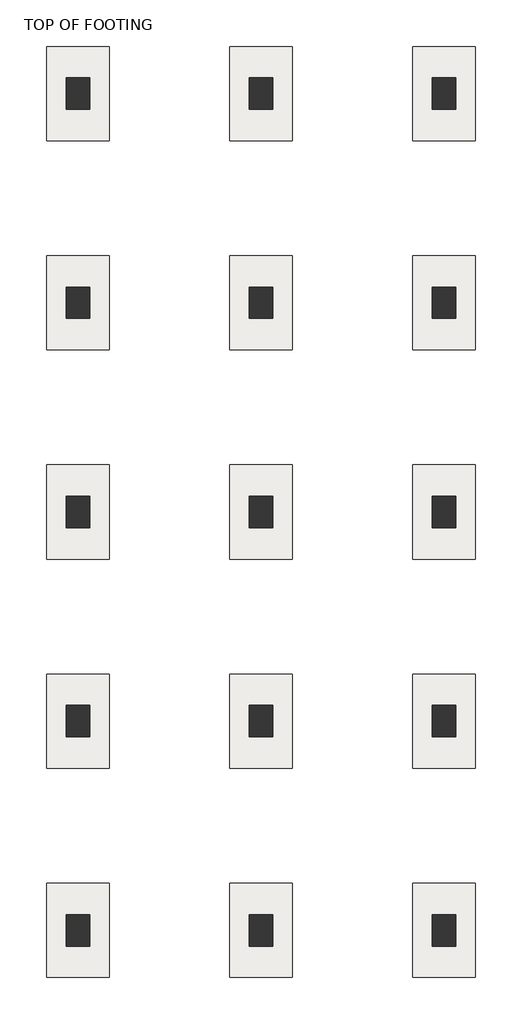
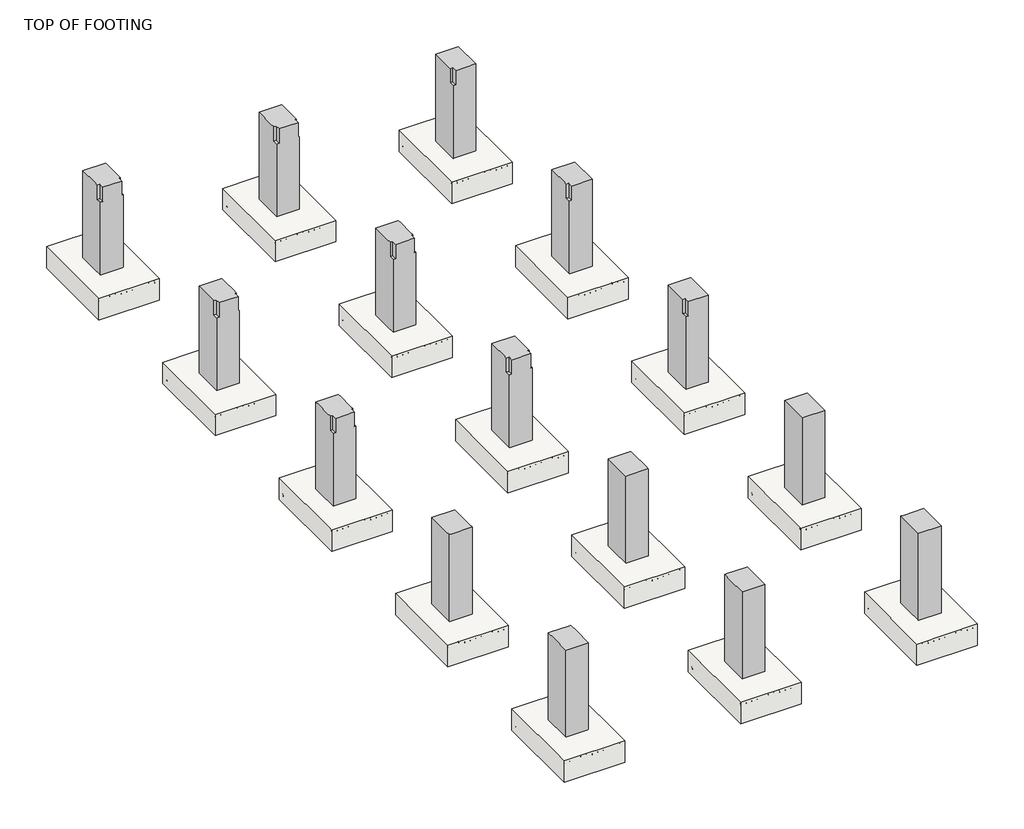
# One storey, part 2 of 11: 15 columns, 15 slabs.
"""IFC4 building model written with IfcOpenShell, lengths in millimetres."""

from ifc_helpers import new_model, si_unit, origin, place, context, project, spatial, faceted_brep, transform, mapped, element, save
from components import m_footing_rectangular_1800_x_1200_x_450mm_16ba7ea5

model = new_model("IFC4")

# Units and contexts
model_context = context("Model", 3, world=origin())
ifc_project = project(units=[si_unit("LENGTHUNIT", "METRE", prefix="MILLI")], contexts=[model_context])

# Site, building, storey
site = spatial("IfcSite", under=ifc_project)
building = spatial("IfcBuilding", under=site)
storey = spatial("IfcBuildingStorey", under=building, Name="TOP OF FOOTING", Elevation=-1828.8)

# Columns
placement = place(None, origin())
element("IfcColumn", 1, ObjectType="M_Concrete-Rectangular-Column : 450 x 600mm", at=placement, inside=storey, context=model_context, shape_type="Brep", body=[
    faceted_brep([(1355.1115906, 19703.1212443, -1828.8), (1355.1115906, 19103.1212443, -1828.8), (905.1115906, 19103.1212443, -1828.8), (905.1115906, 19703.1212443, -1828.8), (1355.1115906, 19703.1212443, 0.0), (1355.1115906, 19303.1212443, 0.0), (1355.1115906, 19203.1212443, 0.0), (1355.1115906, 19203.1212443, -300.0), (1355.1115906, 19103.1212443, -300.0), (1330.1115906, 19103.1212443, -300.0), (1330.1115906, 19103.1212443, 0.0), (955.1115906, 19103.1212443, 0.0), (955.1115906, 19103.1212443, -300.0), (905.1115906, 19103.1212443, -300.0), (905.1115906, 19203.1212443, -300.0), (905.1115906, 19203.1212443, 0.0), (905.1115906, 19303.1212443, 0.0), (905.1115906, 19703.1212443, 0.0), (955.1115906, 19203.1212443, 0.0), (1330.1115906, 19203.1212443, 0.0), (1330.1115906, 19203.1212443, -300.0), (955.1115906, 19203.1212443, -300.0)], [[[0, 1, 2, 3]], [[1, 0, 4, 5, 6, 7, 8]], [[2, 1, 8, 9, 10, 11, 12, 13]], [[3, 2, 13, 14, 15, 16, 17]], [[0, 3, 17, 4]], [[4, 17, 16, 15, 18, 11, 10, 19, 6, 5]], [[7, 20, 9, 8]], [[20, 19, 10, 9]], [[20, 7, 6, 19]], [[21, 14, 13, 12]], [[18, 21, 12, 11]], [[14, 21, 18, 15]]]),
])
element("IfcColumn", 2, ObjectType="M_Concrete-Rectangular-Column : 450 x 600mm", at=placement, inside=storey, context=model_context, shape_type="Brep", body=[
    faceted_brep([(4855.1115906, 19703.1212443, -1828.8), (4855.1115906, 19103.1212443, -1828.8), (4405.1115906, 19103.1212443, -1828.8), (4405.1115906, 19703.1212443, -1828.8), (4855.1115906, 19703.1212443, 0.0), (4855.1115906, 19303.1212443, 0.0), (4855.1115906, 19203.1212443, 0.0), (4855.1115906, 19203.1212443, -300.0), (4855.1115906, 19103.1212443, -300.0), (4830.1115906, 19103.1212443, -300.0), (4830.1115906, 19103.1212443, 0.0), (4455.1115906, 19103.1212443, 0.0), (4455.1115906, 19103.1212443, -300.0), (4405.1115906, 19103.1212443, -300.0), (4405.1115906, 19203.1212443, -300.0), (4405.1115906, 19203.1212443, 0.0), (4405.1115906, 19303.1212443, 0.0), (4405.1115906, 19703.1212443, 0.0), (4455.1115906, 19203.1212443, 0.0), (4830.1115906, 19203.1212443, 0.0), (4830.1115906, 19203.1212443, -300.0), (4455.1115906, 19203.1212443, -300.0)], [[[0, 1, 2, 3]], [[1, 0, 4, 5, 6, 7, 8]], [[2, 1, 8, 9, 10, 11, 12, 13]], [[3, 2, 13, 14, 15, 16, 17]], [[0, 3, 17, 4]], [[4, 17, 16, 15, 18, 11, 10, 19, 6, 5]], [[7, 20, 9, 8]], [[20, 19, 10, 9]], [[20, 7, 6, 19]], [[21, 14, 13, 12]], [[18, 21, 12, 11]], [[14, 21, 18, 15]]]),
])
element("IfcColumn", 3, ObjectType="M_Concrete-Rectangular-Column : 450 x 600mm", at=placement, inside=storey, context=model_context, shape_type="Brep", body=[
    faceted_brep([(8355.1115906, 19703.1212443, -1828.8), (8355.1115906, 19103.1212443, -1828.8), (7905.1115906, 19103.1212443, -1828.8), (7905.1115906, 19703.1212443, -1828.8), (8355.1115906, 19703.1212443, 0.0), (8355.1115906, 19103.1212443, 0.0), (7955.1115906, 19103.1212443, 0.0), (7955.1115906, 19103.1212443, -300.0), (7905.1115906, 19103.1212443, -300.0), (7905.1115906, 19203.1212443, -300.0), (7905.1115906, 19203.1212443, 0.0), (7905.1115906, 19303.1212443, 0.0), (7905.1115906, 19703.1212443, 0.0), (7955.1115906, 19203.1212443, 0.0), (7955.1115906, 19203.1212443, -300.0)], [[[0, 1, 2, 3]], [[1, 0, 4, 5]], [[2, 1, 5, 6, 7, 8]], [[3, 2, 8, 9, 10, 11, 12]], [[0, 3, 12, 4]], [[5, 4, 12, 11, 10, 13, 6]], [[14, 9, 8, 7]], [[13, 14, 7, 6]], [[9, 14, 13, 10]]]),
])
element("IfcColumn", 4, ObjectType="M_Concrete-Rectangular-Column : 450 x 600mm", at=placement, inside=storey, context=model_context, shape_type="Brep", body=[
    faceted_brep([(1355.1115906, 15703.1212443, -1828.8), (1355.1115906, 15103.1212443, -1828.8), (905.1115906, 15103.1212443, -1828.8), (905.1115906, 15703.1212443, -1828.8), (1355.1115906, 15703.1212443, -300.0), (1355.1115906, 15703.1212443, 0.0), (1355.1115906, 15603.1212443, 0.0), (1355.1115906, 15303.1212443, 0.0), (1355.1115906, 15203.1212443, 0.0), (1355.1115906, 15203.1212443, -300.0), (1355.1115906, 15103.1212443, -300.0), (1330.1115906, 15103.1212443, -300.0), (1330.1115906, 15103.1212443, 0.0), (955.1115906, 15103.1212443, 0.0), (955.1115906, 15103.1212443, -300.0), (905.1115906, 15103.1212443, -300.0), (905.1115906, 15203.1212443, -300.0), (905.1115906, 15203.1212443, 0.0), (905.1115906, 15303.1212443, 0.0), (905.1115906, 15603.1212443, 0.0), (905.1115906, 15703.1212443, 0.0), (905.1115906, 15703.1212443, -300.0), (955.1115906, 15203.1212443, 0.0), (1330.1115906, 15203.1212443, 0.0), (1330.1115906, 15203.1212443, -300.0), (955.1115906, 15203.1212443, -300.0)], [[[0, 1, 2, 3]], [[1, 0, 4, 5, 6, 7, 8, 9, 10]], [[2, 1, 10, 11, 12, 13, 14, 15]], [[3, 2, 15, 16, 17, 18, 19, 20, 21]], [[0, 3, 21, 20, 5, 4]], [[5, 20, 19, 18, 17, 22, 13, 12, 23, 8, 7, 6]], [[9, 24, 11, 10]], [[24, 23, 12, 11]], [[24, 9, 8, 23]], [[25, 16, 15, 14]], [[22, 25, 14, 13]], [[16, 25, 22, 17]]]),
])
element("IfcColumn", 5, ObjectType="M_Concrete-Rectangular-Column : 450 x 600mm", at=placement, inside=storey, context=model_context, shape_type="Brep", body=[
    faceted_brep([(4855.1115906, 15703.1212443, -1828.8), (4855.1115906, 15103.1212443, -1828.8), (4405.1115906, 15103.1212443, -1828.8), (4405.1115906, 15703.1212443, -1828.8), (4855.1115906, 15703.1212443, -300.0), (4855.1115906, 15703.1212443, 0.0), (4855.1115906, 15603.1212443, 0.0), (4855.1115906, 15303.1212443, 0.0), (4855.1115906, 15203.1212443, 0.0), (4855.1115906, 15203.1212443, -300.0), (4855.1115906, 15103.1212443, -300.0), (4830.1115906, 15103.1212443, -300.0), (4830.1115906, 15103.1212443, 0.0), (4455.1115906, 15103.1212443, 0.0), (4455.1115906, 15103.1212443, -300.0), (4405.1115906, 15103.1212443, -300.0), (4405.1115906, 15203.1212443, -300.0), (4405.1115906, 15203.1212443, 0.0), (4405.1115906, 15303.1212443, 0.0), (4405.1115906, 15603.1212443, 0.0), (4405.1115906, 15703.1212443, 0.0), (4405.1115906, 15703.1212443, -300.0), (4455.1115906, 15203.1212443, 0.0), (4830.1115906, 15203.1212443, 0.0), (4830.1115906, 15203.1212443, -300.0), (4455.1115906, 15203.1212443, -300.0)], [[[0, 1, 2, 3]], [[1, 0, 4, 5, 6, 7, 8, 9, 10]], [[2, 1, 10, 11, 12, 13, 14, 15]], [[3, 2, 15, 16, 17, 18, 19, 20, 21]], [[0, 3, 21, 20, 5, 4]], [[5, 20, 19, 18, 17, 22, 13, 12, 23, 8, 7, 6]], [[9, 24, 11, 10]], [[24, 23, 12, 11]], [[24, 9, 8, 23]], [[25, 16, 15, 14]], [[22, 25, 14, 13]], [[16, 25, 22, 17]]]),
])
element("IfcColumn", 6, ObjectType="M_Concrete-Rectangular-Column : 450 x 600mm", at=placement, inside=storey, context=model_context, shape_type="Brep", body=[
    faceted_brep([(8355.1115906, 15703.1212443, -1828.8), (8355.1115906, 15103.1212443, -1828.8), (7905.1115906, 15103.1212443, -1828.8), (7905.1115906, 15703.1212443, -1828.8), (8355.1115906, 15703.1212443, 0.0), (8355.1115906, 15103.1212443, 0.0), (7955.1115906, 15103.1212443, 0.0), (7955.1115906, 15103.1212443, -300.0), (7905.1115906, 15103.1212443, -300.0), (7905.1115906, 15203.1212443, -300.0), (7905.1115906, 15203.1212443, 0.0), (7905.1115906, 15303.1212443, 0.0), (7905.1115906, 15603.1212443, 0.0), (7905.1115906, 15703.1212443, 0.0), (7905.1115906, 15703.1212443, -300.0), (7955.1115906, 15203.1212443, 0.0), (7955.1115906, 15203.1212443, -300.0)], [[[0, 1, 2, 3]], [[1, 0, 4, 5]], [[2, 1, 5, 6, 7, 8]], [[3, 2, 8, 9, 10, 11, 12, 13, 14]], [[0, 3, 14, 13, 4]], [[5, 4, 13, 12, 11, 10, 15, 6]], [[16, 9, 8, 7]], [[15, 16, 7, 6]], [[9, 16, 15, 10]]]),
])
element("IfcColumn", 7, ObjectType="M_Concrete-Rectangular-Column : 450 x 600mm", at=placement, inside=storey, context=model_context, shape_type="Brep", body=[
    faceted_brep([(1355.1115906, 11703.1212443, -1828.8), (1355.1115906, 11103.1212443, -1828.8), (905.1115906, 11103.1212443, -1828.8), (905.1115906, 11703.1212443, -1828.8), (1355.1115906, 11703.1212443, -300.0), (1355.1115906, 11703.1212443, 0.0), (1355.1115906, 11603.1212443, 0.0), (1355.1115906, 11303.1212443, 0.0), (1355.1115906, 11203.1212443, 0.0), (1355.1115906, 11203.1212443, -300.0), (1355.1115906, 11103.1212443, -300.0), (1330.1115906, 11103.1212443, -300.0), (1330.1115906, 11103.1212443, 0.0), (955.1115906, 11103.1212443, 0.0), (955.1115906, 11103.1212443, -300.0), (905.1115906, 11103.1212443, -300.0), (905.1115906, 11203.1212443, -300.0), (905.1115906, 11203.1212443, 0.0), (905.1115906, 11303.1212443, 0.0), (905.1115906, 11603.1212443, 0.0), (905.1115906, 11703.1212443, 0.0), (905.1115906, 11703.1212443, -300.0), (955.1115906, 11203.1212443, 0.0), (1330.1115906, 11203.1212443, 0.0), (1330.1115906, 11203.1212443, -300.0), (955.1115906, 11203.1212443, -300.0)], [[[0, 1, 2, 3]], [[1, 0, 4, 5, 6, 7, 8, 9, 10]], [[2, 1, 10, 11, 12, 13, 14, 15]], [[3, 2, 15, 16, 17, 18, 19, 20, 21]], [[0, 3, 21, 20, 5, 4]], [[5, 20, 19, 18, 17, 22, 13, 12, 23, 8, 7, 6]], [[9, 24, 11, 10]], [[24, 23, 12, 11]], [[24, 9, 8, 23]], [[25, 16, 15, 14]], [[22, 25, 14, 13]], [[16, 25, 22, 17]]]),
])
element("IfcColumn", 8, ObjectType="M_Concrete-Rectangular-Column : 450 x 600mm", at=placement, inside=storey, context=model_context, shape_type="Brep", body=[
    faceted_brep([(4855.1115906, 11703.1212443, -1828.8), (4855.1115906, 11103.1212443, -1828.8), (4405.1115906, 11103.1212443, -1828.8), (4405.1115906, 11703.1212443, -1828.8), (4855.1115906, 11703.1212443, -300.0), (4855.1115906, 11703.1212443, 0.0), (4855.1115906, 11603.1212443, 0.0), (4855.1115906, 11303.1212443, 0.0), (4855.1115906, 11203.1212443, 0.0), (4855.1115906, 11203.1212443, -300.0), (4855.1115906, 11103.1212443, -300.0), (4830.1115906, 11103.1212443, -300.0), (4830.1115906, 11103.1212443, 0.0), (4455.1115906, 11103.1212443, 0.0), (4455.1115906, 11103.1212443, -300.0), (4405.1115906, 11103.1212443, -300.0), (4405.1115906, 11203.1212443, -300.0), (4405.1115906, 11203.1212443, 0.0), (4405.1115906, 11303.1212443, 0.0), (4405.1115906, 11603.1212443, 0.0), (4405.1115906, 11703.1212443, 0.0), (4405.1115906, 11703.1212443, -300.0), (4455.1115906, 11203.1212443, 0.0), (4830.1115906, 11203.1212443, 0.0), (4830.1115906, 11203.1212443, -300.0), (4455.1115906, 11203.1212443, -300.0)], [[[0, 1, 2, 3]], [[1, 0, 4, 5, 6, 7, 8, 9, 10]], [[2, 1, 10, 11, 12, 13, 14, 15]], [[3, 2, 15, 16, 17, 18, 19, 20, 21]], [[0, 3, 21, 20, 5, 4]], [[5, 20, 19, 18, 17, 22, 13, 12, 23, 8, 7, 6]], [[9, 24, 11, 10]], [[24, 23, 12, 11]], [[24, 9, 8, 23]], [[25, 16, 15, 14]], [[22, 25, 14, 13]], [[16, 25, 22, 17]]]),
])
element("IfcColumn", 9, ObjectType="M_Concrete-Rectangular-Column : 450 x 600mm", at=placement, inside=storey, context=model_context, shape_type="Brep", body=[
    faceted_brep([(8355.1115906, 11703.1212443, -1828.8), (8355.1115906, 11103.1212443, -1828.8), (7905.1115906, 11103.1212443, -1828.8), (7905.1115906, 11703.1212443, -1828.8), (8355.1115906, 11703.1212443, 0.0), (8355.1115906, 11103.1212443, 0.0), (7955.1115906, 11103.1212443, 0.0), (7955.1115906, 11103.1212443, -300.0), (7905.1115906, 11103.1212443, -300.0), (7905.1115906, 11203.1212443, -300.0), (7905.1115906, 11203.1212443, 0.0), (7905.1115906, 11303.1212443, 0.0), (7905.1115906, 11603.1212443, 0.0), (7905.1115906, 11703.1212443, 0.0), (7905.1115906, 11703.1212443, -300.0), (7955.1115906, 11203.1212443, 0.0), (7955.1115906, 11203.1212443, -300.0)], [[[0, 1, 2, 3]], [[1, 0, 4, 5]], [[2, 1, 5, 6, 7, 8]], [[3, 2, 8, 9, 10, 11, 12, 13, 14]], [[0, 3, 14, 13, 4]], [[5, 4, 13, 12, 11, 10, 15, 6]], [[16, 9, 8, 7]], [[15, 16, 7, 6]], [[9, 16, 15, 10]]]),
])
element("IfcColumn", 10, ObjectType="M_Concrete-Rectangular-Column : 450 x 600mm", at=placement, inside=storey, context=model_context, shape_type="Brep", body=[
    faceted_brep([(1355.1115906, 7703.1212443, -1828.8), (1355.1115906, 7103.1212443, -1828.8), (905.1115906, 7103.1212443, -1828.8), (905.1115906, 7703.1212443, -1828.8), (1355.1115906, 7703.1212443, -300.0), (1355.1115906, 7703.1212443, 0.0), (1355.1115906, 7603.1212443, 0.0), (1355.1115906, 7203.1212443, 0.0), (1355.1115906, 7103.1212443, 0.0), (1355.1115906, 7103.1212443, -300.0), (1330.1115906, 7103.1212443, 0.0), (955.1115906, 7103.1212443, 0.0), (905.1115906, 7103.1212443, 0.0), (905.1115906, 7103.1212443, -300.0), (905.1115906, 7203.1212443, 0.0), (905.1115906, 7603.1212443, 0.0), (905.1115906, 7703.1212443, 0.0), (905.1115906, 7703.1212443, -300.0)], [[[0, 1, 2, 3]], [[1, 0, 4, 5, 6, 7, 8, 9]], [[2, 1, 9, 8, 10, 11, 12, 13]], [[3, 2, 13, 12, 14, 15, 16, 17]], [[0, 3, 17, 16, 5, 4]], [[5, 16, 15, 14, 12, 11, 10, 8, 7, 6]]]),
])
element("IfcColumn", 11, ObjectType="M_Concrete-Rectangular-Column : 450 x 600mm", at=placement, inside=storey, context=model_context, shape_type="Brep", body=[
    faceted_brep([(4855.1115906, 7703.1212443, -1828.8), (4855.1115906, 7103.1212443, -1828.8), (4405.1115906, 7103.1212443, -1828.8), (4405.1115906, 7703.1212443, -1828.8), (4855.1115906, 7703.1212443, -300.0), (4855.1115906, 7703.1212443, 0.0), (4855.1115906, 7603.1212443, 0.0), (4855.1115906, 7203.1212443, 0.0), (4855.1115906, 7103.1212443, 0.0), (4855.1115906, 7103.1212443, -300.0), (4830.1115906, 7103.1212443, 0.0), (4455.1115906, 7103.1212443, 0.0), (4405.1115906, 7103.1212443, 0.0), (4405.1115906, 7103.1212443, -300.0), (4405.1115906, 7203.1212443, 0.0), (4405.1115906, 7603.1212443, 0.0), (4405.1115906, 7703.1212443, 0.0), (4405.1115906, 7703.1212443, -300.0)], [[[0, 1, 2, 3]], [[1, 0, 4, 5, 6, 7, 8, 9]], [[2, 1, 9, 8, 10, 11, 12, 13]], [[3, 2, 13, 12, 14, 15, 16, 17]], [[0, 3, 17, 16, 5, 4]], [[5, 16, 15, 14, 12, 11, 10, 8, 7, 6]]]),
])
element("IfcColumn", 12, ObjectType="M_Concrete-Rectangular-Column : 450 x 600mm", at=placement, inside=storey, context=model_context, shape_type="Brep", body=[
    faceted_brep([(8355.1115906, 7703.1212443, -1828.8), (8355.1115906, 7103.1212443, -1828.8), (7905.1115906, 7103.1212443, -1828.8), (7905.1115906, 7703.1212443, -1828.8), (8355.1115906, 7703.1212443, 0.0), (8355.1115906, 7103.1212443, 0.0), (7955.1115906, 7103.1212443, 0.0), (7905.1115906, 7103.1212443, 0.0), (7905.1115906, 7103.1212443, -300.0), (7905.1115906, 7203.1212443, 0.0), (7905.1115906, 7603.1212443, 0.0), (7905.1115906, 7703.1212443, 0.0), (7905.1115906, 7703.1212443, -300.0)], [[[0, 1, 2, 3]], [[1, 0, 4, 5]], [[2, 1, 5, 6, 7, 8]], [[3, 2, 8, 7, 9, 10, 11, 12]], [[0, 3, 12, 11, 4]], [[5, 4, 11, 10, 9, 7, 6]]]),
])
element("IfcColumn", 13, ObjectType="M_Concrete-Rectangular-Column : 450 x 600mm", at=placement, inside=storey, context=model_context, shape_type="Brep", body=[
    faceted_brep([(1355.1115906, 3703.1212443, -1828.8), (1355.1115906, 3103.1212443, -1828.8), (905.1115906, 3103.1212443, -1828.8), (905.1115906, 3703.1212443, -1828.8), (1355.1115906, 3703.1212443, -300.0), (1355.1115906, 3703.1212443, 0.0), (1355.1115906, 3503.1212443, 0.0), (1355.1115906, 3103.1212443, 0.0), (905.1115906, 3103.1212443, 0.0), (905.1115906, 3503.1212443, 0.0), (905.1115906, 3703.1212443, 0.0), (905.1115906, 3703.1212443, -300.0), (955.1115906, 3703.1212443, 0.0), (1330.1115906, 3703.1212443, 0.0)], [[[0, 1, 2, 3]], [[1, 0, 4, 5, 6, 7]], [[2, 1, 7, 8]], [[3, 2, 8, 9, 10, 11]], [[0, 3, 11, 10, 12, 13, 5, 4]], [[8, 7, 6, 5, 13, 12, 10, 9]]]),
])
element("IfcColumn", 14, ObjectType="M_Concrete-Rectangular-Column : 450 x 600mm", at=placement, inside=storey, context=model_context, shape_type="Brep", body=[
    faceted_brep([(4855.1115906, 3703.1212443, -1828.8), (4855.1115906, 3103.1212443, -1828.8), (4405.1115906, 3103.1212443, -1828.8), (4405.1115906, 3703.1212443, -1828.8), (4855.1115906, 3703.1212443, -300.0), (4855.1115906, 3703.1212443, 0.0), (4855.1115906, 3503.1212443, 0.0), (4855.1115906, 3103.1212443, 0.0), (4405.1115906, 3103.1212443, 0.0), (4405.1115906, 3503.1212443, 0.0), (4405.1115906, 3703.1212443, 0.0), (4405.1115906, 3703.1212443, -300.0), (4455.1115906, 3703.1212443, 0.0), (4830.1115906, 3703.1212443, 0.0)], [[[0, 1, 2, 3]], [[1, 0, 4, 5, 6, 7]], [[2, 1, 7, 8]], [[3, 2, 8, 9, 10, 11]], [[0, 3, 11, 10, 12, 13, 5, 4]], [[8, 7, 6, 5, 13, 12, 10, 9]]]),
])
element("IfcColumn", 15, ObjectType="M_Concrete-Rectangular-Column : 450 x 600mm", at=placement, inside=storey, context=model_context, shape_type="Brep", body=[
    faceted_brep([(8355.1115906, 3703.1212443, -1828.8), (8355.1115906, 3103.1212443, -1828.8), (7905.1115906, 3103.1212443, -1828.8), (7905.1115906, 3703.1212443, -1828.8), (8355.1115906, 3703.1212443, 0.0), (8355.1115906, 3103.1212443, 0.0), (7905.1115906, 3103.1212443, 0.0), (7905.1115906, 3503.1212443, 0.0), (7905.1115906, 3703.1212443, 0.0), (7905.1115906, 3703.1212443, -300.0), (7955.1115906, 3703.1212443, 0.0)], [[[0, 1, 2, 3]], [[1, 0, 4, 5]], [[2, 1, 5, 6]], [[3, 2, 6, 7, 8, 9]], [[0, 3, 9, 8, 10, 4]], [[5, 4, 10, 8, 7, 6]]]),
])

# Slabs
m_footing_rectangular_1800_x_1200_x_450mm_shape = m_footing_rectangular_1800_x_1200_x_450mm_16ba7ea5(model_context)
element("IfcSlab", 16, ObjectType="M_Footing-Rectangular : 1800 x 1200 x 450mm", at=placement, inside=storey, context=model_context, shape_type="MappedRepresentation", body=[
    mapped(m_footing_rectangular_1800_x_1200_x_450mm_shape, transform((1130.1115906, 19403.1212443, -1828.8), x_axis=(1.0, 0.0, 0.0), y_axis=(0.0, 1.0, 0.0), z_axis=(0.0, 0.0, 1.0))),
])
element("IfcSlab", 17, ObjectType="M_Footing-Rectangular : 1800 x 1200 x 450mm", at=placement, inside=storey, context=model_context, shape_type="MappedRepresentation", body=[
    mapped(m_footing_rectangular_1800_x_1200_x_450mm_shape, transform((4630.1115906, 19403.1212443, -1828.8), x_axis=(1.0, 0.0, 0.0), y_axis=(0.0, 1.0, 0.0), z_axis=(0.0, 0.0, 1.0))),
])
element("IfcSlab", 18, ObjectType="M_Footing-Rectangular : 1800 x 1200 x 450mm", at=placement, inside=storey, context=model_context, shape_type="MappedRepresentation", body=[
    mapped(m_footing_rectangular_1800_x_1200_x_450mm_shape, transform((8130.1115906, 19403.1212443, -1828.8), x_axis=(1.0, 0.0, 0.0), y_axis=(0.0, 1.0, 0.0), z_axis=(0.0, 0.0, 1.0))),
])
element("IfcSlab", 19, ObjectType="M_Footing-Rectangular : 1800 x 1200 x 450mm", at=placement, inside=storey, context=model_context, shape_type="MappedRepresentation", body=[
    mapped(m_footing_rectangular_1800_x_1200_x_450mm_shape, transform((1130.1115906, 3403.1212443, -1828.8), x_axis=(1.0, 0.0, 0.0), y_axis=(0.0, 1.0, 0.0), z_axis=(0.0, 0.0, 1.0))),
])
element("IfcSlab", 20, ObjectType="M_Footing-Rectangular : 1800 x 1200 x 450mm", at=placement, inside=storey, context=model_context, shape_type="MappedRepresentation", body=[
    mapped(m_footing_rectangular_1800_x_1200_x_450mm_shape, transform((4630.1115906, 3403.1212443, -1828.8), x_axis=(1.0, 0.0, 0.0), y_axis=(0.0, 1.0, 0.0), z_axis=(0.0, 0.0, 1.0))),
])
element("IfcSlab", 21, ObjectType="M_Footing-Rectangular : 1800 x 1200 x 450mm", at=placement, inside=storey, context=model_context, shape_type="MappedRepresentation", body=[
    mapped(m_footing_rectangular_1800_x_1200_x_450mm_shape, transform((8130.1115906, 3403.1212443, -1828.8), x_axis=(1.0, 0.0, 0.0), y_axis=(0.0, 1.0, 0.0), z_axis=(0.0, 0.0, 1.0))),
])
element("IfcSlab", 22, ObjectType="M_Footing-Rectangular : 1800 x 1200 x 450mm", at=placement, inside=storey, context=model_context, shape_type="MappedRepresentation", body=[
    mapped(m_footing_rectangular_1800_x_1200_x_450mm_shape, transform((8130.1115906, 7403.1212443, -1828.8), x_axis=(1.0, 0.0, 0.0), y_axis=(0.0, 1.0, 0.0), z_axis=(0.0, 0.0, 1.0))),
])
element("IfcSlab", 23, ObjectType="M_Footing-Rectangular : 1800 x 1200 x 450mm", at=placement, inside=storey, context=model_context, shape_type="MappedRepresentation", body=[
    mapped(m_footing_rectangular_1800_x_1200_x_450mm_shape, transform((4630.1115906, 7403.1212443, -1828.8), x_axis=(1.0, 0.0, 0.0), y_axis=(0.0, 1.0, 0.0), z_axis=(0.0, 0.0, 1.0))),
])
element("IfcSlab", 24, ObjectType="M_Footing-Rectangular : 1800 x 1200 x 450mm", at=placement, inside=storey, context=model_context, shape_type="MappedRepresentation", body=[
    mapped(m_footing_rectangular_1800_x_1200_x_450mm_shape, transform((1130.1115906, 7403.1212443, -1828.8), x_axis=(1.0, 0.0, 0.0), y_axis=(0.0, 1.0, 0.0), z_axis=(0.0, 0.0, 1.0))),
])
element("IfcSlab", 25, ObjectType="M_Footing-Rectangular : 1800 x 1200 x 450mm", at=placement, inside=storey, context=model_context, shape_type="MappedRepresentation", body=[
    mapped(m_footing_rectangular_1800_x_1200_x_450mm_shape, transform((1130.1115906, 11403.1212443, -1828.8), x_axis=(1.0, 0.0, 0.0), y_axis=(0.0, 1.0, 0.0), z_axis=(0.0, 0.0, 1.0))),
])
element("IfcSlab", 26, ObjectType="M_Footing-Rectangular : 1800 x 1200 x 450mm", at=placement, inside=storey, context=model_context, shape_type="MappedRepresentation", body=[
    mapped(m_footing_rectangular_1800_x_1200_x_450mm_shape, transform((4630.1115906, 11403.1212443, -1828.8), x_axis=(1.0, 0.0, 0.0), y_axis=(0.0, 1.0, 0.0), z_axis=(0.0, 0.0, 1.0))),
])
element("IfcSlab", 27, ObjectType="M_Footing-Rectangular : 1800 x 1200 x 450mm", at=placement, inside=storey, context=model_context, shape_type="MappedRepresentation", body=[
    mapped(m_footing_rectangular_1800_x_1200_x_450mm_shape, transform((8130.1115906, 11403.1212443, -1828.8), x_axis=(1.0, 0.0, 0.0), y_axis=(0.0, 1.0, 0.0), z_axis=(0.0, 0.0, 1.0))),
])
element("IfcSlab", 28, ObjectType="M_Footing-Rectangular : 1800 x 1200 x 450mm", at=placement, inside=storey, context=model_context, shape_type="MappedRepresentation", body=[
    mapped(m_footing_rectangular_1800_x_1200_x_450mm_shape, transform((8130.1115906, 15403.1212443, -1828.8), x_axis=(1.0, 0.0, 0.0), y_axis=(0.0, 1.0, 0.0), z_axis=(0.0, 0.0, 1.0))),
])
element("IfcSlab", 29, ObjectType="M_Footing-Rectangular : 1800 x 1200 x 450mm", at=placement, inside=storey, context=model_context, shape_type="MappedRepresentation", body=[
    mapped(m_footing_rectangular_1800_x_1200_x_450mm_shape, transform((4630.1115906, 15403.1212443, -1828.8), x_axis=(1.0, 0.0, 0.0), y_axis=(0.0, 1.0, 0.0), z_axis=(0.0, 0.0, 1.0))),
])
element("IfcSlab", 30, ObjectType="M_Footing-Rectangular : 1800 x 1200 x 450mm", at=placement, inside=storey, context=model_context, shape_type="MappedRepresentation", body=[
    mapped(m_footing_rectangular_1800_x_1200_x_450mm_shape, transform((1130.1115906, 15403.1212443, -1828.8), x_axis=(1.0, 0.0, 0.0), y_axis=(0.0, 1.0, 0.0), z_axis=(0.0, 0.0, 1.0))),
])

save(model, "model.ifc")

# Revit data of these elements
# Type "M_Concrete-Rectangular-Column : 450 x 600mm"
#   b = 1' - 5.71654"
#   h = 1' - 11.62205"
#   Structural Material [instance default] = Concrete, Cast-in-Place gray
# Type "M_Footing-Rectangular : 1800 x 1200 x 450mm"
#   Width = 3' - 11.24409"
#   Length = 5' - 10.86614"
#   Foundation Thickness = 1' - 5.71654"
#   Structural Material [instance default] = Concrete, Cast-in-Place gray
#   Assembly Code = ""
# Elements 1, 2, 3, 4, 5, 6, 7, 8, 9, 10, 11, 12, 13, 14, 15 (IfcColumn, "M_Concrete-Rectangular-Column : 450 x 600mm")
#   Structural Material = Concrete, Cast-in-Place gray
#   Phase Created = New Construction
#   Materials on its faces: "Concrete, Cast-in-Place gray"
# Elements 16, 17, 18, 19, 20, 21, 22, 23, 24, 25, 26, 27, 28, 29, 30 (IfcSlab, "M_Footing-Rectangular : 1800 x 1200 x 450mm")
#   Structural Material = Concrete, Cast-in-Place gray
#   Phase Created = New Construction
#   Materials on its faces: "Concrete, Cast-in-Place gray"
# Materials
#   "Concrete, Cast-in-Place gray": class "Concrete", colour RGB 192 192 192, transparency 0, Description = "Cast-in-place concrete", Cost = 0
